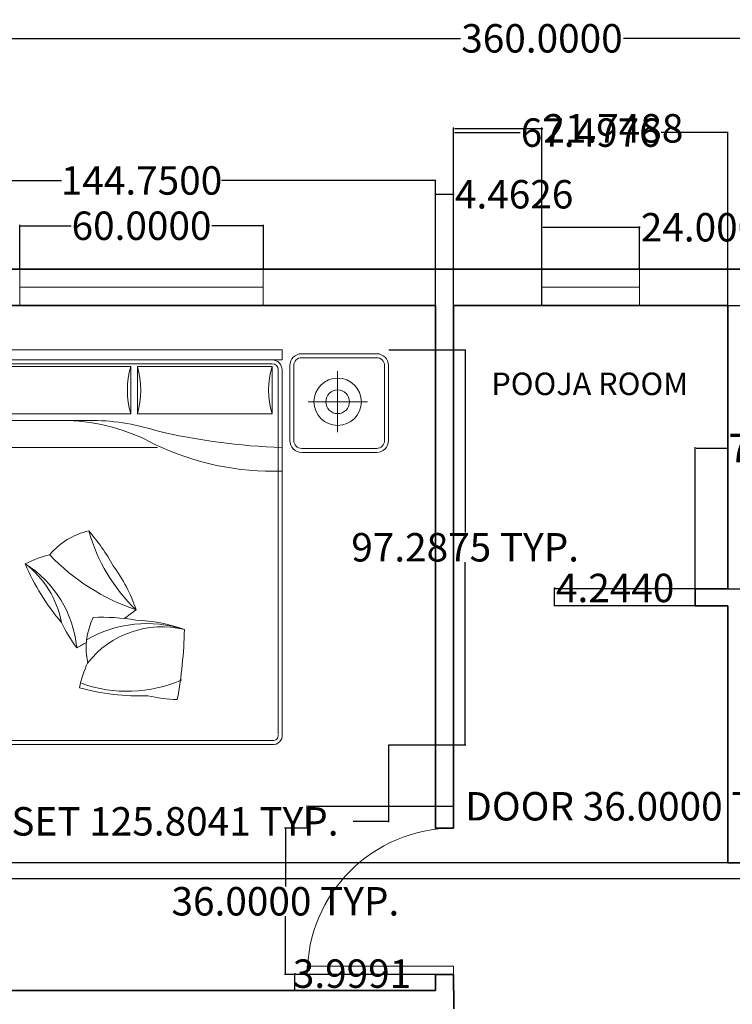
# Model space of a CAD drawing. Units: inches. Extents: x 774 to 2194, y 522 to 1247.
# Tile 5 of 7: x 912 to 1088, y 870 to 1112. Entities that reach past the tile are written whole.
import ezdxf

# ---------------------------------------------------------------- set-up
doc = ezdxf.new("R2010")
doc.units = ezdxf.units.IN
for name, color, linetype, lineweight in [('A-ANNO-DIMS', 2, 'Continuous', 13), ('A-AREA-IDEN', 3, 'Continuous', 18), ('A-DOOR', 3, 'Continuous', 18), ('A-FURN', 8, 'Continuous', 18), ('A-GLAZ', 4, 'Continuous', 18), ('A-WALL', 7, 'Continuous', 35)]:
    doc.layers.add(name, color=color, linetype=linetype, lineweight=lineweight)
doc.styles.get("Standard").update_dxf_attribs({"font": 'arial.ttf'})
doc.dimstyles.get("Standard").update_dxf_attribs({"dimtxt": 7, "dimasz": 0.18, "dimexe": 0.18, "dimexo": 0.0625, "dimgap": 0.09, "dimtad": 0, "dimtih": 1, "dimtoh": 1, "dimdec": 4, "dimzin": 0, "dimdsep": 46, "dimtxsty": 'Standard', "dimcen": 0.09, "dimadec": 0, "dimazin": 0, "dimtfac": 1, "dimtdec": 4, "dimtofl": 0, "dimtmove": 0, "dimatfit": 3, "dimfxl": 1, "dimtolj": 1, "dimtzin": 0, "dimarcsym": 0})

# ---------------------------------------------------------------- blocks, each defined once
blk = doc.blocks.new('A$C356F0359')
for p, q in [((0.5489, 2), (2.0492, 2)), ((0.5489, 1.9489), (0.5489, 2)), ((2.0492, 1.9489), (2.0492, 2)), ((0.4398, 1.9801), (0.0598, 1.9801)), ((0.4398, 1.9601), (0.0598, 1.9601)), ((2.0492, 1.9489), (0.5489, 1.9489)), ((2.5283, 1.9801), (2.1483, 1.9801)), ((2.5283, 1.9601), (2.1483, 1.9601)), ((-0.0002, 1.9201), (-0.0002, 1.5401)), ((0.0198, 1.9201), (0.0198, 1.5401)), ((0.4798, 1.5401), (0.4798, 1.9201)), ((0.4998, 1.5401), (0.4998, 1.9201)), ((0.5489, 1.8977), (0.5489, 0.0512)), ((0.5689, 1.8977), (0.5689, 0.0512)), ((1.998, 1.9289), (0.6001, 1.9289)), ((2.0292, 0.0512), (2.0292, 1.8977)), ((2.0492, 0.0512), (2.0492, 1.8977)), ((2.0883, 1.9201), (2.0883, 1.5401)), ((2.1083, 1.9201), (2.1083, 1.5401)), ((2.5683, 1.5401), (2.5683, 1.9201)), ((2.5883, 1.5401), (2.5883, 1.9201)), ((0.1539, 1.5681), (0.1539, 1.8777)), ((0.2725, 1.8879), (0.2702, 1.8856)), ((0.2702, 1.8856), (0.2702, 1.7279)), ((0.2725, 1.8879), (0.4531, 1.8879)), ((0.3913, 1.8753), (0.277, 1.8753)), ((0.277, 1.8753), (0.277, 1.8147)), ((0.3913, 1.8147), (0.3913, 1.8753)), ((0.4016, 1.8787), (0.4062, 1.8845)), ((0.4016, 1.7404), (0.4016, 1.8787)), ((0.4062, 1.881), (0.405, 1.8765)), ((0.405, 1.8765), (0.4153, 1.8662)), ((0.405, 1.8765), (0.405, 1.8456)), ((0.4062, 1.8845), (0.4405, 1.8845)), ((0.4108, 1.8833), (0.4062, 1.881)), ((0.4108, 1.8833), (0.4382, 1.8833)), ((0.4165, 1.8685), (0.4108, 1.8833)), ((0.4153, 1.8662), (0.4165, 1.8685)), ((0.4153, 1.8147), (0.4153, 1.8662)), ((0.4325, 1.8685), (0.4165, 1.8685)), ((0.4325, 1.8685), (0.4382, 1.8833)), ((0.4336, 1.8662), (0.4325, 1.8685)), ((0.4439, 1.8765), (0.4336, 1.8662)), ((0.4336, 1.8147), (0.4336, 1.8662)), ((0.4382, 1.8833), (0.4428, 1.881)), ((0.4405, 1.8845), (0.4462, 1.8787)), ((0.4428, 1.881), (0.4439, 1.8765)), ((0.4439, 1.8765), (0.4439, 1.8456)), ((0.4462, 1.8787), (0.4462, 1.7416)), ((0.4531, 1.8879), (0.4553, 1.8856)), ((0.4553, 1.8856), (0.4553, 1.7279)), ((2.3306, 1.5822), (2.3306, 1.8917)), ((0.277, 1.8147), (0.3913, 1.8147)), ((0.3913, 1.8125), (0.2816, 1.8125)), ((0.2816, 1.8125), (0.2816, 1.801)), ((0.2816, 1.801), (0.3913, 1.801)), ((0.2907, 1.8125), (0.2907, 1.801)), ((0.2999, 1.8125), (0.2999, 1.801)), ((0.309, 1.8125), (0.309, 1.801)), ((0.3182, 1.8125), (0.3182, 1.801)), ((0.3273, 1.8125), (0.3273, 1.801)), ((0.3365, 1.8125), (0.3365, 1.801)), ((0.3913, 1.801), (0.3913, 1.8125)), ((0.405, 1.8456), (0.4073, 1.8399)), ((0.4073, 1.8399), (0.4108, 1.8342)), ((0.4108, 1.8342), (0.4119, 1.8262)), ((0.4119, 1.8262), (0.4119, 1.8147)), ((0.4119, 1.793), (0.4119, 1.8147)), ((0.4153, 1.8147), (0.4153, 1.753)), ((0.4336, 1.8147), (0.4336, 1.753)), ((0.4382, 1.8342), (0.4371, 1.8262)), ((0.4371, 1.8262), (0.4371, 1.8147)), ((0.4371, 1.793), (0.4371, 1.8147)), ((0.4416, 1.8399), (0.4382, 1.8342)), ((0.4439, 1.8456), (0.4416, 1.8399)), ((0.277, 1.7885), (0.277, 1.7679)), ((0.3445, 1.7885), (0.277, 1.7885)), ((0.277, 1.7679), (0.3445, 1.7679)), ((0.2782, 1.7622), (0.2782, 1.7576)), ((0.2896, 1.7622), (0.2782, 1.7622)), ((0.2782, 1.7576), (0.2896, 1.7576)), ((0.2885, 1.7862), (0.2885, 1.7827)), ((0.2919, 1.7862), (0.2885, 1.7862)), ((0.2885, 1.7827), (0.2919, 1.7827)), ((0.2919, 1.7736), (0.2885, 1.7736)), ((0.2885, 1.7736), (0.2885, 1.7702)), ((0.2885, 1.7702), (0.2919, 1.7702)), ((0.2896, 1.7576), (0.2896, 1.7622)), ((0.2919, 1.7827), (0.2919, 1.7862)), ((0.2919, 1.7702), (0.2919, 1.7736)), ((0.2942, 1.7622), (0.2942, 1.7576)), ((0.3056, 1.7622), (0.2942, 1.7622)), ((0.2942, 1.7576), (0.3056, 1.7576)), ((0.3056, 1.7576), (0.3056, 1.7622)), ((0.3125, 1.7862), (0.309, 1.7862)), ((0.309, 1.7862), (0.309, 1.7827)), ((0.309, 1.7827), (0.3125, 1.7827)), ((0.3125, 1.7736), (0.309, 1.7736)), ((0.309, 1.7736), (0.309, 1.7702)), ((0.309, 1.7702), (0.3125, 1.7702)), ((0.3102, 1.7622), (0.3102, 1.7576)), ((0.3216, 1.7622), (0.3102, 1.7622)), ((0.3102, 1.7576), (0.3216, 1.7576)), ((0.3125, 1.7827), (0.3125, 1.7862)), ((0.3125, 1.7702), (0.3125, 1.7736)), ((0.3216, 1.7576), (0.3216, 1.7622)), ((0.3376, 1.7622), (0.3262, 1.7622)), ((0.3262, 1.7622), (0.3262, 1.7576)), ((0.3262, 1.7576), (0.3376, 1.7576)), ((0.333, 1.7862), (0.3296, 1.7862)), ((0.3296, 1.7862), (0.3296, 1.7827)), ((0.3296, 1.7827), (0.333, 1.7827)), ((0.333, 1.7736), (0.3296, 1.7736)), ((0.3296, 1.7736), (0.3296, 1.7702)), ((0.3296, 1.7702), (0.333, 1.7702)), ((0.333, 1.7827), (0.333, 1.7862)), ((0.333, 1.7702), (0.333, 1.7736)), ((0.3376, 1.7576), (0.3376, 1.7622)), ((0.3445, 1.7679), (0.3445, 1.7885)), ((0.3548, 1.7759), (0.3548, 1.7827)), ((0.3548, 1.7827), (0.3639, 1.7827)), ((0.3639, 1.7759), (0.3548, 1.7759)), ((0.3548, 1.7633), (0.3548, 1.7702)), ((0.3548, 1.7702), (0.3639, 1.7702)), ((0.3639, 1.7633), (0.3548, 1.7633)), ((0.3548, 1.7564), (0.3639, 1.7564)), ((0.3548, 1.7496), (0.3548, 1.7564)), ((0.3639, 1.7496), (0.3548, 1.7496)), ((0.3639, 1.7827), (0.3639, 1.7759)), ((0.3639, 1.7702), (0.3639, 1.7633)), ((0.3639, 1.7564), (0.3639, 1.7496)), ((0.3685, 1.7827), (0.3776, 1.7827)), ((0.3685, 1.7759), (0.3685, 1.7827)), ((0.3776, 1.7759), (0.3685, 1.7759)), ((0.3685, 1.7633), (0.3685, 1.7702)), ((0.3685, 1.7702), (0.3776, 1.7702)), ((0.3776, 1.7633), (0.3685, 1.7633)), ((0.3685, 1.7564), (0.3776, 1.7564)), ((0.3685, 1.7496), (0.3685, 1.7564)), ((0.3776, 1.7496), (0.3685, 1.7496)), ((0.3776, 1.7827), (0.3776, 1.7759)), ((0.3776, 1.7702), (0.3776, 1.7633)), ((0.3776, 1.7564), (0.3776, 1.7496)), ((0.3822, 1.7759), (0.3822, 1.7827)), ((0.3822, 1.7827), (0.3913, 1.7827)), ((0.3913, 1.7759), (0.3822, 1.7759)), ((0.3822, 1.7633), (0.3822, 1.7702)), ((0.3822, 1.7702), (0.3913, 1.7702)), ((0.3913, 1.7633), (0.3822, 1.7633)), ((0.3822, 1.7576), (0.3913, 1.7576)), ((0.3822, 1.7507), (0.3822, 1.7576)), ((0.3913, 1.7507), (0.3822, 1.7507)), ((0.3913, 1.7827), (0.3913, 1.7759)), ((0.3913, 1.7702), (0.3913, 1.7633)), ((0.3913, 1.7576), (0.3913, 1.7507)), ((0.405, 1.7736), (0.4073, 1.7793)), ((0.405, 1.7427), (0.405, 1.7736)), ((0.405, 1.7427), (0.4153, 1.753)), ((0.4073, 1.7793), (0.4108, 1.785)), ((0.4108, 1.785), (0.4119, 1.793)), ((0.4165, 1.7507), (0.4108, 1.7359)), ((0.4153, 1.753), (0.4165, 1.7507)), ((0.4325, 1.7507), (0.4165, 1.7507)), ((0.4336, 1.753), (0.4325, 1.7507)), ((0.4325, 1.7507), (0.4382, 1.7359)), ((0.4439, 1.7427), (0.4336, 1.753)), ((0.4382, 1.785), (0.4371, 1.793)), ((0.4416, 1.7793), (0.4382, 1.785)), ((0.4439, 1.7736), (0.4416, 1.7793)), ((0.4439, 1.7427), (0.4439, 1.7736)), ((0.4622, 1.7459), (0.4553, 1.7484)), ((0.3052, 1.7226), (0.0051, 1.7226)), ((0.2702, 1.7279), (0.2725, 1.7256)), ((0.4244, 1.7256), (0.2725, 1.7256)), ((0.2782, 1.745), (0.2896, 1.745)), ((0.2782, 1.7382), (0.2782, 1.745)), ((0.2896, 1.7382), (0.2782, 1.7382)), ((0.2896, 1.745), (0.2896, 1.7382)), ((0.2942, 1.745), (0.3056, 1.745)), ((0.2942, 1.7382), (0.2942, 1.745)), ((0.3056, 1.7382), (0.2942, 1.7382)), ((0.3056, 1.745), (0.3056, 1.7382)), ((0.3102, 1.745), (0.3216, 1.745)), ((0.3102, 1.7382), (0.3102, 1.745)), ((0.3216, 1.7382), (0.3102, 1.7382)), ((0.3216, 1.745), (0.3216, 1.7382)), ((0.3262, 1.7382), (0.3262, 1.745)), ((0.3262, 1.745), (0.3376, 1.745)), ((0.3376, 1.7382), (0.3262, 1.7382)), ((0.3376, 1.745), (0.3376, 1.7382)), ((0.3548, 1.737), (0.3548, 1.7439)), ((0.3548, 1.7439), (0.3639, 1.7439)), ((0.3639, 1.737), (0.3548, 1.737)), ((0.3639, 1.7439), (0.3639, 1.737)), ((0.3685, 1.737), (0.3685, 1.7439)), ((0.3685, 1.7439), (0.3776, 1.7439)), ((0.3776, 1.737), (0.3685, 1.737)), ((0.3776, 1.7439), (0.3776, 1.737)), ((0.3822, 1.7439), (0.3913, 1.7439)), ((0.3822, 1.737), (0.3822, 1.7439)), ((0.3913, 1.737), (0.3822, 1.737)), ((0.3913, 1.7439), (0.3913, 1.737)), ((0.4073, 1.7347), (0.4016, 1.7404)), ((0.4062, 1.7382), (0.405, 1.7427)), ((0.4108, 1.7359), (0.4062, 1.7382)), ((0.4234, 1.7347), (0.4073, 1.7347)), ((0.4108, 1.7359), (0.4234, 1.7359)), ((0.4233, 1.7393), (0.4235, 1.7294)), ((0.4268, 1.7393), (0.4233, 1.7393)), ((0.4235, 1.7294), (0.4263, 1.7179)), ((0.4263, 1.7179), (0.429, 1.707)), ((0.427, 1.697), (0.4265, 1.6915)), ((0.4274, 1.7301), (0.4268, 1.7393)), ((0.427, 1.7359), (0.4382, 1.7359)), ((0.4295, 1.6996), (0.427, 1.697)), ((0.4405, 1.7347), (0.4271, 1.7347)), ((0.429, 1.7227), (0.4274, 1.7301)), ((0.4531, 1.7256), (0.4284, 1.7256)), ((0.429, 1.707), (0.4288, 1.701)), ((0.4288, 1.701), (0.4295, 1.6996)), ((0.4318, 1.7119), (0.429, 1.7227)), ((0.4325, 1.7063), (0.4318, 1.7119)), ((0.4323, 1.7003), (0.4325, 1.7063)), ((0.4364, 1.6973), (0.4323, 1.7003)), ((0.4355, 1.6919), (0.4364, 1.6973)), ((0.4382, 1.7359), (0.4428, 1.7382)), ((0.4462, 1.7416), (0.4405, 1.7347)), ((0.4428, 1.7382), (0.4439, 1.7427)), ((0.4553, 1.7279), (0.4531, 1.7256)), ((0.4553, 1.7439), (0.4604, 1.7425)), ((0.4604, 1.7425), (0.465, 1.7388)), ((0.4654, 1.7427), (0.4622, 1.7459)), ((0.465, 1.7388), (0.4662, 1.7372)), ((0.4678, 1.7405), (0.4654, 1.7427)), ((0.4662, 1.7372), (0.4686, 1.7374)), ((0.4686, 1.7374), (0.4662, 1.735)), ((0.4662, 1.735), (0.4755, 1.7268)), ((0.4721, 1.7421), (0.4678, 1.7405)), ((0.4741, 1.7401), (0.4721, 1.7421)), ((0.4725, 1.7366), (0.4741, 1.7401)), ((0.4753, 1.7388), (0.4725, 1.7366)), ((0.4783, 1.7356), (0.4753, 1.7388)), ((0.4755, 1.7268), (0.4906, 1.7139)), ((0.4759, 1.729), (0.4783, 1.7356)), ((0.4821, 1.7322), (0.4759, 1.729)), ((0.4874, 1.7272), (0.4821, 1.7322)), ((0.4862, 1.7199), (0.4874, 1.7272)), ((0.4914, 1.7231), (0.4862, 1.7199)), ((0.4908, 1.7135), (0.4984, 1.6917)), ((0.4958, 1.7185), (0.4914, 1.7231)), ((0.494, 1.7135), (0.4958, 1.7185)), ((0.501, 1.7142), (0.494, 1.7135)), ((0.4964, 1.7047), (0.5031, 1.7072)), ((0.5038, 1.7049), (0.4964, 1.7047)), ((0.5005, 1.695), (0.5054, 1.6996)), ((0.5031, 1.7072), (0.501, 1.7142)), ((0.5054, 1.6996), (0.5038, 1.7049)), ((2.4819, 1.7366), (2.1818, 1.7366)), ((0.4265, 1.6915), (0.4332, 1.6903)), ((0.4332, 1.6903), (0.4267, 1.6864)), ((0.4267, 1.6864), (0.4272, 1.6801)), ((0.4272, 1.6801), (0.4346, 1.6794)), ((0.4346, 1.6794), (0.4281, 1.6744)), ((0.4281, 1.6744), (0.4311, 1.669)), ((0.4311, 1.669), (0.4381, 1.6704)), ((0.4381, 1.6704), (0.4348, 1.6639)), ((0.4348, 1.6639), (0.4383, 1.6598)), ((0.4367, 1.6774), (0.4355, 1.6919)), ((0.4455, 1.6663), (0.4367, 1.6774)), ((0.4383, 1.6598), (0.4436, 1.6637)), ((0.4436, 1.6637), (0.4427, 1.6575)), ((0.4427, 1.6575), (0.4471, 1.6547)), ((0.4577, 1.6598), (0.4455, 1.6663)), ((0.4471, 1.6547), (0.4526, 1.6593)), ((0.4526, 1.6593), (0.4519, 1.6517)), ((0.4519, 1.6517), (0.4568, 1.6503)), ((0.4568, 1.6503), (0.4598, 1.6565)), ((0.4716, 1.6586), (0.4577, 1.6598)), ((0.4598, 1.6565), (0.4626, 1.6503)), ((0.4626, 1.6503), (0.4665, 1.6498)), ((0.4665, 1.6498), (0.4681, 1.6565)), ((0.4681, 1.6565), (0.4707, 1.6491)), ((0.4707, 1.6491), (0.4751, 1.6503)), ((0.485, 1.6644), (0.4716, 1.6586)), ((0.4751, 1.6503), (0.4753, 1.6565)), ((0.4753, 1.6565), (0.4806, 1.6519)), ((0.4806, 1.6519), (0.4843, 1.6538)), ((0.4843, 1.6538), (0.4836, 1.6607)), ((0.4836, 1.6607), (0.4885, 1.6547)), ((0.4952, 1.6744), (0.485, 1.6644)), ((0.4885, 1.6547), (0.4922, 1.6579)), ((0.4922, 1.6579), (0.4894, 1.6642)), ((0.4894, 1.6642), (0.4959, 1.6614)), ((0.4984, 1.6917), (0.4952, 1.6744)), ((0.4957, 1.6704), (0.5024, 1.6683)), ((0.4989, 1.6642), (0.4957, 1.6704)), ((0.4959, 1.6614), (0.4989, 1.6642)), ((0.5042, 1.673), (0.4987, 1.6792)), ((0.4987, 1.6792), (0.5058, 1.679)), ((0.5068, 1.695), (0.5005, 1.695)), ((0.5008, 1.6871), (0.5079, 1.6892)), ((0.5068, 1.6836), (0.5008, 1.6871)), ((0.5024, 1.6683), (0.5042, 1.673)), ((0.5058, 1.679), (0.5068, 1.6836)), ((0.5079, 1.6892), (0.5068, 1.695)), ((0.0598, 1.5001), (0.4398, 1.5001)), ((2.1483, 1.5001), (2.5283, 1.5001)), ((0.0598, 1.4801), (0.4398, 1.4801)), ((2.1483, 1.4801), (2.5283, 1.4801)), ((0.6001, 0.02), (1.998, 0.02)), ((0.6001, 0), (1.998, 0))]:
    blk.add_line(p, q)
at = {"linetype": 'ByBlock'}
for p, q in [((0.6001, 1.9147), (1.282, 1.9147)), ((0.6001, 1.6759), (0.6001, 1.9147)), ((1.282, 1.9147), (1.282, 1.6759)), ((1.3161, 1.9147), (1.998, 1.9147)), ((1.3161, 1.6759), (1.3161, 1.9147)), ((1.998, 1.9147), (1.998, 1.6759)), ((1.282, 1.6759), (0.6001, 1.6759)), ((1.998, 1.6759), (1.3161, 1.6759)), ((1.0687, 1.6418), (0.5489, 1.6418)), ((1.4185, 1.5053), (0.5489, 1.5053))]:
    blk.add_line(p, q, dxfattribs=at)
for centre in [(2.3306, 1.7366), (0.1539, 1.7226)]:
    blk.add_circle(centre, 0.12, dxfattribs=at)
for centre in [(2.3306, 1.7366), (0.1539, 1.7226)]:
    blk.add_circle(centre, 0.06)
for centre, radius, start, end in [((0.0598, 1.9201), 0.06, 90, 180), ((0.0598, 1.9201), 0.04, 90, 180), ((0.4398, 1.9201), 0.06, 0, 90), ((0.4398, 1.9201), 0.04, 0, 90), ((0.6001, 1.8977), 0.0512, 90, 180), ((1.998, 1.8977), 0.0512, 0, 90), ((2.1483, 1.9201), 0.06, 90, 180), ((2.1483, 1.9201), 0.04, 90, 180), ((2.5283, 1.9201), 0.06, 0, 90), ((2.5283, 1.9201), 0.04, 0, 90), ((0.6001, 1.8977), 0.0312, 90, 180), ((1.998, 1.8977), 0.0312, 0, 90), ((0.0598, 1.5401), 0.06, 180, 270), ((0.0598, 1.5401), 0.04, 180, 270), ((0.4398, 1.5401), 0.04, 270, 0), ((0.4398, 1.5401), 0.06, 270, 0), ((2.1483, 1.5401), 0.06, 180, 270), ((2.1483, 1.5401), 0.04, 180, 270), ((2.5283, 1.5401), 0.06, 270, 0), ((2.5283, 1.5401), 0.04, 270, 0), ((1.1471, 0.7332), 0.3575, 102.4782, 140.4625), ((1.9086, 1.3124), 0.8697, 195.336, 226.4193), ((0.3249, 0.4335), 0.9879, 28.4971, 41.0566), ((0.9965, 0.4273), 0.548, 103.2034, 117.0362), ((1.6529, 1.7059), 1.0798, 223.6306, 251.4288), ((0.4451, 0.4375), 0.5655, 5.3391, 57.6895), ((0.4517, 0.5274), 0.4879, 10.6986, 52.6864), ((1.8195, 1.3719), 1.1652, 203.0642, 220.3209), ((0.5617, 0.4344), 0.7874, 18.3527, 36.6851), ((-0.021, 2.4319), 2.1977, 305.2966, 307.2418), ((1.5949, 0.9312), 0.734, 205.259, 216.9351), ((1.4135, 0.487), 0.3575, 154.0418, 192.0262), ((1.3641, 0.0041), 0.6085, 71.81, 120.1351), ((1.1372, -0.3434), 0.9879, 80.0607, 92.6202), ((1.2836, -0.1573), 0.7874, 69.9163, 88.2487), ((1.44, 0.1186), 0.4774, 76.1849, 142.0017), ((-0.6432, 0.628), 2.1977, 349.4884, 358.8054), ((-0.021, 2.4319), 2.1977, 297.9248, 299.3793), ((1.5595, 0.1789), 0.548, 154.767, 168.5998), ((1.2647, 0.9578), 0.6885, 250.2936, 293.6414), ((1.3312, 1.4107), 1.1652, 254.6278, 271.8845), ((1.5368, 0.9609), 0.734, 256.8226, 268.4988), ((0.5943, 0.0454), 0.0458, 172.7599, 277.2401), ((2.0038, 0.0454), 0.0458, 262.7599, 7.2401), ((0.5943, 0.0454), 0.0258, 172.7599, 277.2401), ((2.0038, 0.0454), 0.0258, 262.7599, 7.2401)]:
    blk.add_arc(centre, radius, start, end)
for centre, radius, start, end in [((0.1906, 1.7953), 0.4265, 343.7398, 16.2602), ((1.6914, 1.7953), 0.4265, 163.7398, 196.2602), ((0.9067, 1.7953), 0.4265, 343.7398, 16.2602), ((2.4075, 1.7953), 0.4265, 163.7398, 196.2602), ((0.9303, 0.657), 0.9853, 61.4328, 88.1261), ((1.0826, 0.5712), 1.0706, 72.1966, 90.7418), ((2.1368, 4.5996), 3.0955, 256.4201, 268.3789), ((2.0056, 2.7745), 1.3903, 244.2427, 271.7984)]:
    blk.add_arc(centre, radius, start, end, dxfattribs=at)
blk = doc.blocks.new('*D7')
at = {"layer": 'A-ANNO-DIMS', "color": 0, "lineweight": -2, "transparency": 16777216}
for p, q in [((912.16, 1050.75), (912.16, 1061.53)), ((912.34, 1061.35), (924.81, 1061.35)), ((971.98, 1061.35), (959.5, 1061.35)), ((972.16, 1050.75), (972.16, 1061.53))]:
    blk.add_line(p, q, dxfattribs=at)
at = {"layer": 'A-ANNO-DIMS', "color": 0, "transparency": 16777216}
for points in [[(912.34, 1061.38), (912.34, 1061.32), (912.16, 1061.35)], [(971.98, 1061.38), (971.98, 1061.32), (972.16, 1061.35)]]:
    blk.add_solid(points, dxfattribs=at)
at = {"layer": 'Defpoints', "color": 0, "transparency": 16777216}
for p in [(972.16, 1061.35), (912.16, 1050.69), (972.16, 1050.69)]:
    blk.add_point(p, dxfattribs=at)
at = {"layer": 'A-ANNO-DIMS', "color": 0, "transparency": 16777216, "insert": (942.16, 1061.35), "char_height": 7, "attachment_point": 5}
blk.add_mtext('\\A1;60.0000', dxfattribs=at)
blk = doc.blocks.new('*D8')
at = {"layer": 'A-ANNO-DIMS', "color": 0, "lineweight": -2, "transparency": 16777216}
for p, q in [((1040.78, 1050.75), (1040.78, 1061.15)), ((1040.96, 1060.97), (1064.6, 1060.97)), ((1064.78, 1050.75), (1064.78, 1061.15)), ((1064.78, 1060.97), (1064.96, 1060.97))]:
    blk.add_line(p, q, dxfattribs=at)
at = {"layer": 'A-ANNO-DIMS', "color": 0, "transparency": 16777216}
for points in [[(1040.96, 1061), (1040.96, 1060.94), (1040.78, 1060.97)], [(1064.6, 1061), (1064.6, 1060.94), (1064.78, 1060.97)]]:
    blk.add_solid(points, dxfattribs=at)
at = {"layer": 'Defpoints', "color": 0, "transparency": 16777216}
for p in [(1064.78, 1060.97), (1040.78, 1050.69), (1064.78, 1050.69)]:
    blk.add_point(p, dxfattribs=at)
at = {"layer": 'A-ANNO-DIMS', "color": 0, "transparency": 16777216, "insert": (1082.35, 1060.97), "char_height": 7, "attachment_point": 5}
blk.add_mtext('\\A1;24.0000', dxfattribs=at)
blk = doc.blocks.new('*D10')
at = {"layer": 'A-ANNO-DIMS', "color": 0, "lineweight": -2, "transparency": 16777216}
for p, q in [((869.78, 1041.75), (869.78, 1072.68)), ((869.96, 1072.5), (922.44, 1072.5)), ((1014.35, 1072.5), (961.87, 1072.5)), ((1014.53, 1041.75), (1014.53, 1072.68))]:
    blk.add_line(p, q, dxfattribs=at)
at = {"layer": 'A-ANNO-DIMS', "color": 0, "transparency": 16777216}
for points in [[(869.96, 1072.53), (869.96, 1072.47), (869.78, 1072.5)], [(1014.35, 1072.53), (1014.35, 1072.47), (1014.53, 1072.5)]]:
    blk.add_solid(points, dxfattribs=at)
at = {"layer": 'Defpoints', "color": 0, "transparency": 16777216}
for p in [(1014.53, 1072.5), (869.78, 1041.69), (1014.53, 1041.69)]:
    blk.add_point(p, dxfattribs=at)
at = {"layer": 'A-ANNO-DIMS', "color": 0, "transparency": 16777216, "insert": (942.16, 1072.5), "char_height": 7, "attachment_point": 5}
blk.add_mtext('\\A1;144.7500', dxfattribs=at)
blk = doc.blocks.new('*D11')
at = {"layer": 'A-ANNO-DIMS', "color": 0, "lineweight": -2, "transparency": 16777216}
for p, q in [((1014.53, 1041.75), (1014.53, 1069.28)), ((1014.71, 1069.1), (1018.81, 1069.1)), ((1018.99, 1041.75), (1018.99, 1069.28)), ((1018.99, 1069.1), (1019.17, 1069.1))]:
    blk.add_line(p, q, dxfattribs=at)
at = {"layer": 'A-ANNO-DIMS', "color": 0, "transparency": 16777216}
for points in [[(1014.71, 1069.13), (1014.71, 1069.07), (1014.53, 1069.1)], [(1018.81, 1069.13), (1018.81, 1069.07), (1018.99, 1069.1)]]:
    blk.add_solid(points, dxfattribs=at)
at = {"layer": 'Defpoints', "color": 0, "transparency": 16777216}
for p in [(1018.99, 1069.1), (1014.53, 1041.69), (1018.99, 1041.69)]:
    blk.add_point(p, dxfattribs=at)
at = {"layer": 'A-ANNO-DIMS', "color": 0, "transparency": 16777216, "insert": (1033.93, 1069.1), "char_height": 7, "attachment_point": 5}
blk.add_mtext('\\A1;4.4626', dxfattribs=at)
blk = doc.blocks.new('*D12')
at = {"layer": 'A-ANNO-DIMS', "color": 0, "lineweight": -2, "transparency": 16777216}
for p, q in [((1019.03, 1041.75), (1019.03, 1084.47)), ((1019.21, 1084.29), (1035.43, 1084.29)), ((1086.35, 1084.29), (1070.14, 1084.29)), ((1086.53, 1041.75), (1086.53, 1084.47))]:
    blk.add_line(p, q, dxfattribs=at)
at = {"layer": 'A-ANNO-DIMS', "color": 0, "transparency": 16777216}
for points in [[(1019.21, 1084.32), (1019.21, 1084.26), (1019.03, 1084.29)], [(1086.35, 1084.32), (1086.35, 1084.26), (1086.53, 1084.29)]]:
    blk.add_solid(points, dxfattribs=at)
at = {"layer": 'Defpoints', "color": 0, "transparency": 16777216}
for p in [(1086.53, 1084.29), (1019.03, 1041.69), (1086.53, 1041.69)]:
    blk.add_point(p, dxfattribs=at)
at = {"layer": 'A-ANNO-DIMS', "color": 0, "transparency": 16777216, "insert": (1052.78, 1084.29), "char_height": 7, "attachment_point": 5}
blk.add_mtext('\\A1;67.4976', dxfattribs=at)
blk = doc.blocks.new('*D15')
at = {"layer": 'A-ANNO-DIMS', "color": 0, "lineweight": -2, "transparency": 16777216}
for p, q in [((860.78, 1053.45), (860.78, 1107.69)), ((860.96, 1107.51), (1020.74, 1107.51)), ((1220.6, 1107.51), (1060.83, 1107.51)), ((1220.78, 1050.75), (1220.78, 1107.69))]:
    blk.add_line(p, q, dxfattribs=at)
at = {"layer": 'A-ANNO-DIMS', "color": 0, "transparency": 16777216}
for points in [[(860.96, 1107.54), (860.96, 1107.48), (860.78, 1107.51)], [(1220.6, 1107.54), (1220.6, 1107.48), (1220.78, 1107.51)]]:
    blk.add_solid(points, dxfattribs=at)
at = {"layer": 'Defpoints', "color": 0, "transparency": 16777216}
for p in [(1220.78, 1107.51), (860.78, 1053.39), (1220.78, 1050.69)]:
    blk.add_point(p, dxfattribs=at)
at = {"layer": 'A-ANNO-DIMS', "color": 0, "transparency": 16777216, "insert": (1040.78, 1107.51), "char_height": 7, "attachment_point": 5}
blk.add_mtext('\\A1;360.0000', dxfattribs=at)
blk = doc.blocks.new('DOOR-SWING-36IN')
blk.add_line((36, 0), (36, 2))
blk.add_lwpolyline([(36, 2), (0, 2), (0, 0), (36, 0)], close=True)
blk.add_arc((36, 0), 36, 90, 180)
blk = doc.blocks.new('WIN-60IN-EXT')
for p, q in [((0, 0), (0, 9)), ((60, 0), (60, 9)), ((0, 4.5), (60, 4.5))]:
    blk.add_line(p, q)
blk = doc.blocks.new('WIN-24IN-EXT')
for p, q in [((0, 0), (0, 9)), ((24, 0), (24, 9)), ((0, 4.5), (24, 4.5))]:
    blk.add_line(p, q)
blk = doc.blocks.new('*D40')
at = {"layer": 'A-ANNO-DIMS', "color": 0, "lineweight": -2, "transparency": 16777216}
for p, q in [((982.99, 913), (982.99, 918.52)), ((983.17, 918.34), (1018.81, 918.34)), ((1018.99, 913), (1018.99, 918.52)), ((1018.99, 918.34), (1019.17, 918.34))]:
    blk.add_line(p, q, dxfattribs=at)
at = {"layer": 'A-ANNO-DIMS', "color": 0, "transparency": 16777216}
for points in [[(983.17, 918.37), (983.17, 918.31), (982.99, 918.34)], [(1018.81, 918.37), (1018.81, 918.31), (1018.99, 918.34)]]:
    blk.add_solid(points, dxfattribs=at)
at = {"layer": 'Defpoints', "color": 0, "transparency": 16777216}
for p in [(1018.99, 918.34), (982.99, 912.94), (1018.99, 912.94)]:
    blk.add_point(p, dxfattribs=at)
at = {"layer": 'A-ANNO-DIMS', "color": 0, "transparency": 16777216, "insert": (1064.39, 918.34), "char_height": 7, "attachment_point": 5}
blk.add_mtext('\\A1;DOOR 36.0000 TYP.', dxfattribs=at)
blk = doc.blocks.new('*D41')
at = {"layer": 'A-ANNO-DIMS', "color": 0, "lineweight": -2, "transparency": 16777216}
for p, q in [((982.93, 912.94), (977.41, 912.94)), ((977.59, 912.76), (977.59, 898.6)), ((977.59, 877.12), (977.59, 891.27)), ((982.93, 876.94), (977.41, 876.94))]:
    blk.add_line(p, q, dxfattribs=at)
at = {"layer": 'A-ANNO-DIMS', "color": 0, "transparency": 16777216}
for points in [[(977.56, 912.76), (977.62, 912.76), (977.59, 912.94)], [(977.56, 877.12), (977.62, 877.12), (977.59, 876.94)]]:
    blk.add_solid(points, dxfattribs=at)
at = {"layer": 'Defpoints', "color": 0, "transparency": 16777216}
for p in [(977.59, 912.94), (982.99, 912.94), (982.99, 876.94)]:
    blk.add_point(p, dxfattribs=at)
at = {"layer": 'A-ANNO-DIMS', "color": 0, "transparency": 16777216, "insert": (977.59, 894.94), "char_height": 7, "attachment_point": 5}
blk.add_mtext('\\A1;36.0000 TYP.', dxfattribs=at)
blk = doc.blocks.new('*D42')
at = {"layer": 'A-ANNO-DIMS', "color": 0, "lineweight": -2, "transparency": 16777216}
for p, q in [((877.18, 933.44), (877.18, 914.45)), ((1002.99, 933.44), (1002.99, 914.45)), ((877.36, 914.63), (885.88, 914.63)), ((1002.81, 914.63), (994.29, 914.63))]:
    blk.add_line(p, q, dxfattribs=at)
at = {"layer": 'A-ANNO-DIMS', "color": 0, "transparency": 16777216}
for points in [[(877.36, 914.66), (877.36, 914.6), (877.18, 914.63)], [(1002.81, 914.66), (1002.81, 914.6), (1002.99, 914.63)]]:
    blk.add_solid(points, dxfattribs=at)
at = {"layer": 'Defpoints', "color": 0, "transparency": 16777216}
for p in [(877.18, 933.5), (1002.99, 933.5), (1002.99, 914.63)]:
    blk.add_point(p, dxfattribs=at)
at = {"layer": 'A-ANNO-DIMS', "color": 0, "transparency": 16777216, "insert": (940.09, 914.63), "char_height": 7, "attachment_point": 5}
blk.add_mtext('\\A1;BED SET 125.8041 TYP.', dxfattribs=at)
blk = doc.blocks.new('*D43')
at = {"layer": 'A-ANNO-DIMS', "color": 0, "lineweight": -2, "transparency": 16777216}
for p, q in [((1003.05, 1030.79), (1022.04, 1030.79)), ((1021.86, 1030.61), (1021.86, 985.81)), ((1021.86, 933.68), (1021.86, 978.48)), ((1003.05, 933.5), (1022.04, 933.5))]:
    blk.add_line(p, q, dxfattribs=at)
at = {"layer": 'A-ANNO-DIMS', "color": 0, "transparency": 16777216}
for points in [[(1021.83, 1030.61), (1021.89, 1030.61), (1021.86, 1030.79)], [(1021.83, 933.68), (1021.89, 933.68), (1021.86, 933.5)]]:
    blk.add_solid(points, dxfattribs=at)
at = {"layer": 'Defpoints', "color": 0, "transparency": 16777216}
for p in [(1002.99, 1030.79), (1021.86, 1030.79), (1002.99, 933.5)]:
    blk.add_point(p, dxfattribs=at)
at = {"layer": 'A-ANNO-DIMS', "color": 0, "transparency": 16777216, "insert": (1021.86, 982.14), "char_height": 7, "attachment_point": 5}
blk.add_mtext('\\A1;97.2875 TYP.', dxfattribs=at)
blk = doc.blocks.new('*D59')
at = {"layer": 'A-ANNO-DIMS', "color": 0, "lineweight": -2, "transparency": 16777216}
for p, q in [((1019.03, 1041.75), (1019.03, 1085.52)), ((1019.21, 1085.34), (1040.6, 1085.34)), ((1040.78, 1041.75), (1040.78, 1085.52)), ((1040.78, 1085.34), (1040.96, 1085.34))]:
    blk.add_line(p, q, dxfattribs=at)
at = {"layer": 'A-ANNO-DIMS', "color": 0, "transparency": 16777216}
for points in [[(1019.21, 1085.37), (1019.21, 1085.31), (1019.03, 1085.34)], [(1040.6, 1085.37), (1040.6, 1085.31), (1040.78, 1085.34)]]:
    blk.add_solid(points, dxfattribs=at)
at = {"layer": 'Defpoints', "color": 0, "transparency": 16777216}
for p in [(1040.78, 1085.34), (1019.03, 1041.69), (1040.78, 1041.69)]:
    blk.add_point(p, dxfattribs=at)
at = {"layer": 'A-ANNO-DIMS', "color": 0, "transparency": 16777216, "insert": (1058.37, 1085.34), "char_height": 7, "attachment_point": 5}
blk.add_mtext('\\A1;21.7488', dxfattribs=at)
blk = doc.blocks.new('*D72')
at = {"layer": 'A-ANNO-DIMS', "color": 0, "lineweight": -2, "transparency": 16777216}
for p, q in [((1138.97, 904.44), (825.95, 904.44)), ((826.13, 904.44), (826.13, 904.62)), ((826.13, 904.62), (826.31, 904.62)), ((826.13, 900.62), (826.13, 904.26)), ((1138.97, 900.44), (825.95, 900.44))]:
    blk.add_line(p, q, dxfattribs=at)
at = {"layer": 'A-ANNO-DIMS', "color": 0, "transparency": 16777216}
for points in [[(826.1, 904.26), (826.16, 904.26), (826.13, 904.44)], [(826.1, 900.62), (826.16, 900.62), (826.13, 900.44)]]:
    blk.add_solid(points, dxfattribs=at)
at = {"layer": 'Defpoints', "color": 0, "transparency": 16777216}
for p in [(826.13, 904.44), (1139.03, 904.44), (1139.03, 900.44)]:
    blk.add_point(p, dxfattribs=at)
at = {"layer": 'A-ANNO-DIMS', "color": 0, "transparency": 16777216, "insert": (841.06, 904.62), "char_height": 7, "attachment_point": 5}
blk.add_mtext('\\A1;4.0000', dxfattribs=at)
blk = doc.blocks.new('*D73')
at = {"layer": 'A-ANNO-DIMS', "color": 0, "lineweight": -2, "transparency": 16777216}
for p, q in [((1014.47, 876.94), (979.7, 876.94)), ((979.88, 876.94), (979.88, 877.12)), ((979.88, 877.12), (980.06, 877.12)), ((979.88, 873.12), (979.88, 876.76)), ((1014.47, 872.94), (979.7, 872.94))]:
    blk.add_line(p, q, dxfattribs=at)
at = {"layer": 'A-ANNO-DIMS', "color": 0, "transparency": 16777216}
for points in [[(979.85, 876.76), (979.91, 876.76), (979.88, 876.94)], [(979.85, 873.12), (979.91, 873.12), (979.88, 872.94)]]:
    blk.add_solid(points, dxfattribs=at)
at = {"layer": 'Defpoints', "color": 0, "transparency": 16777216}
for p in [(979.88, 876.94), (1014.53, 876.94), (1014.53, 872.94)]:
    blk.add_point(p, dxfattribs=at)
at = {"layer": 'A-ANNO-DIMS', "color": 0, "transparency": 16777216, "insert": (994, 877.12), "char_height": 7, "attachment_point": 5}
blk.add_mtext('\\A1;3.9991', dxfattribs=at)
blk = doc.blocks.new('*D75')
at = {"layer": 'A-ANNO-DIMS', "color": 0, "lineweight": -2, "transparency": 16777216}
for p, q in [((1078.54, 972), (1078.54, 1006.77)), ((1078.72, 1006.59), (1086.35, 1006.59)), ((1086.53, 972), (1086.53, 1006.77)), ((1086.53, 1006.59), (1086.71, 1006.59))]:
    blk.add_line(p, q, dxfattribs=at)
at = {"layer": 'A-ANNO-DIMS', "color": 0, "transparency": 16777216}
for points in [[(1078.72, 1006.62), (1078.72, 1006.56), (1078.54, 1006.59)], [(1086.35, 1006.62), (1086.35, 1006.56), (1086.53, 1006.59)]]:
    blk.add_solid(points, dxfattribs=at)
at = {"layer": 'Defpoints', "color": 0, "transparency": 16777216}
for p in [(1086.53, 1006.59), (1078.54, 971.94), (1086.53, 971.94)]:
    blk.add_point(p, dxfattribs=at)
at = {"layer": 'A-ANNO-DIMS', "color": 0, "transparency": 16777216, "insert": (1101.31, 1006.59), "char_height": 7, "attachment_point": 5}
blk.add_mtext('\\A1;7.9959', dxfattribs=at)
blk = doc.blocks.new('*D76')
at = {"layer": 'A-ANNO-DIMS', "color": 0, "lineweight": -2, "transparency": 16777216}
for p, q in [((1078.47, 971.94), (1043.71, 971.94)), ((1043.89, 971.94), (1043.89, 972.12)), ((1043.89, 972.12), (1044.07, 972.12)), ((1043.89, 967.87), (1043.89, 971.76)), ((1078.47, 967.69), (1043.71, 967.69))]:
    blk.add_line(p, q, dxfattribs=at)
at = {"layer": 'A-ANNO-DIMS', "color": 0, "transparency": 16777216}
for points in [[(1043.86, 971.76), (1043.92, 971.76), (1043.89, 971.94)], [(1043.86, 967.87), (1043.92, 967.87), (1043.89, 967.69)]]:
    blk.add_solid(points, dxfattribs=at)
at = {"layer": 'Defpoints', "color": 0, "transparency": 16777216}
for p in [(1043.89, 971.94), (1078.54, 971.94), (1078.54, 967.69)]:
    blk.add_point(p, dxfattribs=at)
at = {"layer": 'A-ANNO-DIMS', "color": 0, "transparency": 16777216, "insert": (1058.81, 972.12), "char_height": 7, "attachment_point": 5}
blk.add_mtext('\\A1;4.2440', dxfattribs=at)
blk = doc.blocks.new('*D77')
at = {"layer": 'A-ANNO-DIMS', "color": 0, "lineweight": -2, "transparency": 16777216}
for p, q in [((1086.59, 1041.69), (1121.36, 1041.69)), ((1121.18, 1041.51), (1121.18, 1010.48)), ((1121.18, 972.12), (1121.18, 1003.15)), ((1086.59, 971.94), (1121.36, 971.94))]:
    blk.add_line(p, q, dxfattribs=at)
at = {"layer": 'A-ANNO-DIMS', "color": 0, "transparency": 16777216}
for points in [[(1121.15, 1041.51), (1121.21, 1041.51), (1121.18, 1041.69)], [(1121.15, 972.12), (1121.21, 972.12), (1121.18, 971.94)]]:
    blk.add_solid(points, dxfattribs=at)
at = {"layer": 'Defpoints', "color": 0, "transparency": 16777216}
for p in [(1086.53, 1041.69), (1086.53, 971.94), (1121.18, 971.94)]:
    blk.add_point(p, dxfattribs=at)
at = {"layer": 'A-ANNO-DIMS', "color": 0, "transparency": 16777216, "insert": (1121.18, 1006.81), "char_height": 7, "attachment_point": 5}
blk.add_mtext('\\A1;69.7500', dxfattribs=at)

msp = doc.modelspace()

# ---------------------------------------------------------------- linework, layer by layer
at = {"layer": 'A-WALL'}
for p, q in [((1220.78103, 1050.6875), (860.78103, 1050.6875)), ((860.78103, 1050.6875), (1220.78103, 1050.6875)), ((869.78103, 1041.6875), (1014.53103, 1041.6875)), ((869.78103, 1041.6875), (1014.53103, 1041.6875)), ((1014.53103, 1041.6875), (869.78103, 1041.6875)), ((1014.53103, 1041.6875), (1014.53103, 912.93658)), ((1018.99358, 1041.6875), (1086.53103, 1041.6875)), ((1018.99358, 912.93658), (1018.99358, 1041.6875)), ((1018.99358, 1041.6875), (1086.53103, 1041.6875)), ((1086.53103, 1041.6875), (1018.99358, 1041.6875)), ((1019.03347, 1041.6875), (1086.53103, 1041.6875)), ((1086.53103, 1041.6875), (1086.53103, 971.9375)), ((1019.03103, 971.9375), (1019.05243, 971.9375)), ((1078.53512, 971.9375), (1078.53512, 967.69348)), ((1078.53512, 971.9375), (1086.53103, 971.9375)), ((1019.03103, 967.4375), (1019.05366, 967.4375)), ((1078.53512, 967.69348), (1086.53103, 967.69348)), ((1086.53103, 967.69348), (1086.53103, 967.4375)), ((1086.53103, 967.69348), (1086.53103, 904.4375)), ((1014.44527, 912.93658), (1018.99358, 912.93658)), ((1086.53103, 904.4375), (1091.03103, 904.4375)), ((1014.44527, 876.93658), (1018.99358, 876.93658)), ((1014.53103, 876.93658), (1014.53103, 872.9375)), ((1018.99358, 876.93658), (1018.99358, 872.9375)), ((869.78103, 872.9375), (1014.53103, 872.9375)), ((1018.99358, 872.9375), (1019.07934, 872.9375)), ((1019.07934, 872.9375), (1019.08056, 868.4375))]:
    msp.add_line(p, q, dxfattribs=at)

# ---------------------------------------------------------------- block references
at = {"layer": 'A-DOOR'}
msp.add_blockref('DOOR-SWING-36IN', (982.994, 876.937), dxfattribs=at)
at = {"layer": 'A-FURN', "xscale": 48.60038017161549, "yscale": 48.60038017161549, "zscale": 48.60038017161549}
msp.add_blockref('A$C356F0359', (877.19418, 933.58323), dxfattribs=at)
at = {"layer": 'A-GLAZ'}
for name, p in [('WIN-60IN-EXT', (912.156, 1041.688)), ('WIN-24IN-EXT', (1040.782, 1041.688))]:
    msp.add_blockref(name, p, dxfattribs=at)

# ---------------------------------------------------------------- texts
at = {"layer": 'A-AREA-IDEN', "insert": (1028.30576, 1025.1702), "char_height": 5.53791, "attachment_point": 1}
msp.add_mtext('POOJA ROOM', dxfattribs=at)

# ---------------------------------------------------------------- dimensions: what is measured, and where the dimension line sits
at = {"layer": 'A-ANNO-DIMS'}
for base, p1, p2, override, picture, middle in [((1220.78103, 1107.50884), (860.78103, 1053.38824), (1220.78103, 1050.6875), {"dimclrd": 0, "dimclre": 0, "dimclrt": 0}, '*D15', (1040.78103, 1107.50884)), ((1040.78225, 1085.3375), (1019.03347, 1041.6875), (1040.78225, 1041.6875), {"dimdec": 4, "dimlfac": 1, "dimrnd": 0, "dimzin": 0, "dimdsep": 46, "dimlunit": 2}, '*D59', (1058.36842, 1085.3375)), ((1086.53103, 1084.289), (1019.03347, 1041.6875), (1086.53103, 1041.6875), {"dimclrd": 0, "dimclre": 0, "dimclrt": 0}, '*D12', (1052.78225, 1084.289)), ((1014.53103, 1072.49891), (869.78103, 1041.6875), (1014.53103, 1041.6875), {"dimclrd": 0, "dimclre": 0, "dimclrt": 0}, '*D10', (942.15603, 1072.49891)), ((1018.993582, 1069.098875), (1014.531027, 1041.687503), (1018.993582, 1041.687503), {"dimclrd": 0, "dimclre": 0, "dimclrt": 0}, '*D11', (1033.932067, 1069.098875)), ((972.15603, 1061.34572), (912.15603, 1050.6875), (972.15603, 1050.6875), {"dimclrd": 0, "dimclre": 0, "dimclrt": 0}, '*D7', (942.15603, 1061.34572)), ((1064.78225, 1060.97203), (1040.78225, 1050.6875), (1064.78225, 1050.6875), {"dimclrd": 0, "dimclre": 0, "dimclrt": 0}, '*D8', (1082.34932, 1060.97203)), ((1086.53103, 1006.5875), (1078.53512, 971.9375), (1086.53103, 971.9375), {"dimdec": 4, "dimlfac": 1, "dimrnd": 0, "dimzin": 0, "dimdsep": 46, "dimlunit": 2}, '*D75', (1101.30955, 1006.5875))]:
    dim = msp.add_linear_dim(base=base, p1=p1, p2=p2, dimstyle='Standard', override=override, dxfattribs=at)
    dim.commit()
    dim.dimension.update_dxf_attribs({"geometry": picture, "text_midpoint": middle})
for base, p1, p2, angle, picture, middle in [((1121.18103, 971.9375), (1086.53103, 1041.6875), (1086.53103, 971.9375), 270, '*D77', (1121.18103, 1006.8125)), ((1043.88512, 971.9375), (1078.53512, 967.69348), (1078.53512, 971.9375), 90, '*D76', (1058.81406, 972.1175)), ((826.13103, 904.4375), (1139.03103, 900.4375), (1139.03103, 904.4375), 90, '*D72', (841.05996, 904.6175)), ((979.88103, 876.93658), (1014.53103, 872.9375), (1014.53103, 876.93658), 90, '*D73', (994.00301, 877.11658))]:
    dim = msp.add_linear_dim(base=base, p1=p1, p2=p2, angle=angle, dimstyle='Standard', override={"dimdec": 4, "dimlfac": 1, "dimrnd": 0, "dimzin": 0, "dimdsep": 46, "dimlunit": 2}, dxfattribs=at)
    dim.commit()
    dim.dimension.update_dxf_attribs({"geometry": picture, "text_midpoint": middle})
for base, p1, p2, picture, middle in [((1021.85788, 1030.78583), (1002.98727, 933.49835), (1002.98727, 1030.78583), '*D43', (1021.85788, 982.14209)), ((977.59358, 912.93658), (982.99358, 876.93658), (982.99358, 912.93658), '*D41', (977.59358, 894.93658))]:
    dim = msp.add_linear_dim(base=base, p1=p1, p2=p2, angle=90, text='<> TYP.', dimstyle='Standard', override={"dimdec": 4, "dimlfac": 1, "dimrnd": 0, "dimzin": 0, "dimdsep": 46, "dimlunit": 2}, dxfattribs=at)
    dim.commit()
    dim.dimension.update_dxf_attribs({"geometry": picture, "text_midpoint": middle})
for base, p1, p2, text, picture, middle in [((1002.98727, 914.62773), (877.18318, 933.49835), (1002.98727, 933.49835), 'BED SET <> TYP.', '*D42', (940.08523, 914.62773)), ((1018.99358, 918.33658), (982.99358, 912.93658), (1018.99358, 912.93658), 'DOOR <> TYP.', '*D40', (1064.38875, 918.33658))]:
    dim = msp.add_linear_dim(base=base, p1=p1, p2=p2, text=text, dimstyle='Standard', override={"dimdec": 4, "dimlfac": 1, "dimrnd": 0, "dimzin": 0, "dimdsep": 46, "dimlunit": 2}, dxfattribs=at)
    dim.commit()
    dim.dimension.update_dxf_attribs({"geometry": picture, "text_midpoint": middle})

doc.saveas('drawing.dxf')
